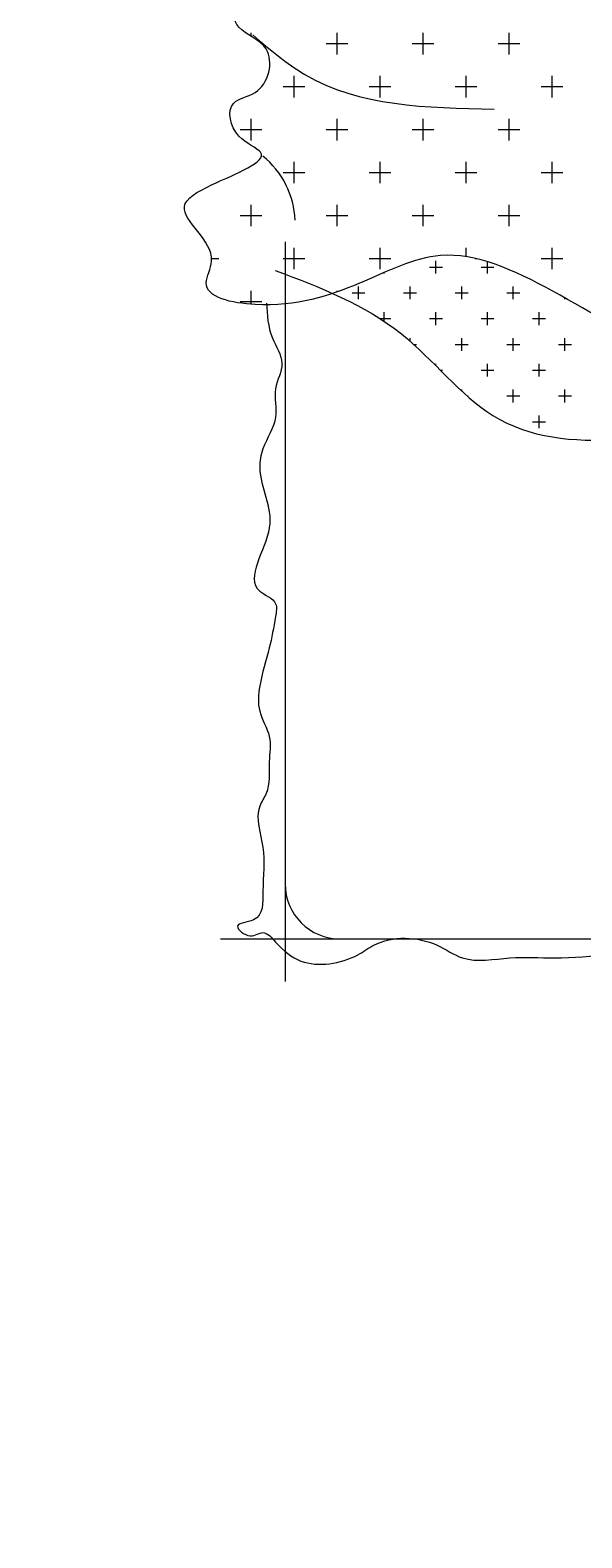
# Model space of a CAD drawing. Units: inches. Extents: x 2330 to 3943, y 1763 to 3461.
# Tile 15 of 40: x 3106 to 3148, y 2547 to 2662. Entities that reach past the tile are written whole.
import ezdxf

# ---------------------------------------------------------------- set-up
doc = ezdxf.new("R2010")
doc.units = ezdxf.units.IN
doc.layers.add('A-ANNO-DIMS', color=2, linetype='Continuous', lineweight=18)
doc.layers.add('A-FURN', color=8, linetype='Continuous', lineweight=13)
doc.styles.get("Standard").update_dxf_attribs({"font": 'arial.ttf'})
doc.dimstyles.get("Standard").update_dxf_attribs({"dimtxt": 0.18, "dimasz": 0.18, "dimexe": 0.18, "dimexo": 0.0625, "dimgap": 0.09, "dimtad": 0, "dimtih": 1, "dimtoh": 1, "dimdec": 4, "dimzin": 0, "dimdsep": 46, "dimtxsty": 'Standard', "dimcen": 0.09, "dimadec": 0, "dimazin": 0, "dimtfac": 1, "dimtdec": 4, "dimtofl": 0, "dimtmove": 0, "dimatfit": 3, "dimfxl": 1, "dimtolj": 1, "dimtzin": 0, "dimarcsym": 0})

# ---------------------------------------------------------------- blocks, each defined once
blk = doc.blocks.new('A$C200C7901')
for p, q in [((0.4504, 1.6834), (0.4504, 1.6883)), ((0.4504, 1.6834), (0.4504, 1.6883)), ((0.4656, 1.6727), (0.466, 1.6727)), ((0.4656, 1.6727), (0.466, 1.6727)), ((0.5597, 1.6727), (0.591, 1.6727)), ((0.5597, 1.6727), (0.591, 1.6727)), ((0.4504, 1.532), (0.4504, 1.5633)), ((0.4347, 1.5477), (0.466, 1.5477)), ((0.6847, 1.5477), (0.716, 1.5477)), ((0.4347, 1.4227), (0.466, 1.4227)), ((0.5, 1.3845), (0.5, 0.3086)), ((0.3931, 1.3602), (0.4035, 1.3602)), ((0.3931, 1.3602), (0.4035, 1.3602)), ((0.4972, 1.3602), (0.5285, 1.3602)), ((0.4972, 1.3602), (0.5285, 1.3602)), ((0.4347, 1.2977), (0.466, 1.2977)), ((0.4347, 1.2977), (0.466, 1.2977)), ((0.4504, 1.2936), (0.4504, 1.3133)), ((0.4504, 1.2936), (0.4504, 1.3133)), ((0.4061, 0.3703), (2.0386, 0.3703))]:
    blk.add_line(p, q)
at = {"linetype": 'ByBlock'}
for p, q in [((0.5754, 1.657), (0.5754, 1.6883)), ((0.5754, 1.657), (0.5754, 1.6883)), ((0.6847, 1.6727), (0.716, 1.6727)), ((0.6847, 1.6727), (0.716, 1.6727)), ((0.7004, 1.657), (0.7004, 1.6883)), ((0.7004, 1.657), (0.7004, 1.6883)), ((0.8097, 1.6727), (0.841, 1.6727)), ((0.8097, 1.6727), (0.841, 1.6727)), ((0.8254, 1.657), (0.8254, 1.6883)), ((0.8254, 1.657), (0.8254, 1.6883)), ((0.5129, 1.5945), (0.5129, 1.6258)), ((0.5129, 1.5945), (0.5129, 1.6258)), ((0.6379, 1.5945), (0.6379, 1.6258)), ((0.6379, 1.5945), (0.6379, 1.6258)), ((0.7629, 1.5945), (0.7629, 1.6258)), ((0.7629, 1.5945), (0.7629, 1.6258)), ((0.8879, 1.5945), (0.8879, 1.6258)), ((0.8879, 1.5945), (0.8879, 1.6258)), ((0.4972, 1.6102), (0.5285, 1.6102)), ((0.4972, 1.6102), (0.5285, 1.6102)), ((0.6222, 1.6102), (0.6535, 1.6102)), ((0.6222, 1.6102), (0.6535, 1.6102)), ((0.7472, 1.6102), (0.7785, 1.6102)), ((0.7472, 1.6102), (0.7785, 1.6102)), ((0.8722, 1.6102), (0.9035, 1.6102)), ((0.8722, 1.6102), (0.9035, 1.6102)), ((0.4504, 1.532), (0.4504, 1.5633)), ((0.5754, 1.532), (0.5754, 1.5633)), ((0.5754, 1.532), (0.5754, 1.5633)), ((0.7004, 1.532), (0.7004, 1.5633)), ((0.7004, 1.532), (0.7004, 1.5633)), ((0.8254, 1.532), (0.8254, 1.5633)), ((0.8254, 1.532), (0.8254, 1.5633)), ((0.4347, 1.5477), (0.466, 1.5477)), ((0.5597, 1.5477), (0.591, 1.5477)), ((0.5597, 1.5477), (0.591, 1.5477)), ((0.6847, 1.5477), (0.716, 1.5477)), ((0.8097, 1.5477), (0.841, 1.5477)), ((0.8097, 1.5477), (0.841, 1.5477)), ((0.5129, 1.4695), (0.5129, 1.5008)), ((0.5129, 1.4695), (0.5129, 1.5008)), ((0.6379, 1.4695), (0.6379, 1.5008)), ((0.6379, 1.4695), (0.6379, 1.5008)), ((0.7629, 1.4695), (0.7629, 1.5008)), ((0.7629, 1.4695), (0.7629, 1.5008)), ((0.8879, 1.4695), (0.8879, 1.5008)), ((0.8879, 1.4695), (0.8879, 1.5008)), ((0.4972, 1.4852), (0.5285, 1.4852)), ((0.4972, 1.4852), (0.5285, 1.4852)), ((0.6222, 1.4852), (0.6535, 1.4852)), ((0.6222, 1.4852), (0.6535, 1.4852)), ((0.7472, 1.4852), (0.7785, 1.4852)), ((0.7472, 1.4852), (0.7785, 1.4852)), ((0.8722, 1.4852), (0.9035, 1.4852)), ((0.8722, 1.4852), (0.9035, 1.4852)), ((0.4504, 1.407), (0.4504, 1.4383)), ((0.4504, 1.407), (0.4504, 1.4383)), ((0.5754, 1.407), (0.5754, 1.4383)), ((0.5754, 1.407), (0.5754, 1.4383)), ((0.7004, 1.407), (0.7004, 1.4383)), ((0.7004, 1.407), (0.7004, 1.4383)), ((0.8254, 1.407), (0.8254, 1.4383)), ((0.8254, 1.407), (0.8254, 1.4383)), ((0.4347, 1.4227), (0.466, 1.4227)), ((0.5597, 1.4227), (0.591, 1.4227)), ((0.5597, 1.4227), (0.591, 1.4227)), ((0.6847, 1.4227), (0.716, 1.4227)), ((0.6847, 1.4227), (0.716, 1.4227)), ((0.8097, 1.4227), (0.841, 1.4227)), ((0.8097, 1.4227), (0.841, 1.4227)), ((0.5129, 1.3445), (0.5129, 1.3758)), ((0.5129, 1.3445), (0.5129, 1.3758)), ((0.6222, 1.3602), (0.6535, 1.3602)), ((0.6222, 1.3602), (0.6535, 1.3602)), ((0.6379, 1.3445), (0.6379, 1.3758)), ((0.6379, 1.3445), (0.6379, 1.3758)), ((0.7629, 1.3627), (0.7629, 1.3758)), ((0.7629, 1.3627), (0.7629, 1.3758)), ((0.7762, 1.3602), (0.7785, 1.3602)), ((0.7762, 1.3602), (0.7785, 1.3602)), ((0.8722, 1.3602), (0.9035, 1.3602)), ((0.8722, 1.3602), (0.9035, 1.3602)), ((0.8879, 1.3445), (0.8879, 1.3758)), ((0.8879, 1.3445), (0.8879, 1.3758)), ((0.6441, 1.3383), (0.6441, 1.3399)), ((0.6441, 1.3383), (0.6441, 1.3399)), ((0.7097, 1.3477), (0.7285, 1.3477)), ((0.7097, 1.3477), (0.7285, 1.3477)), ((0.7191, 1.3383), (0.7191, 1.357)), ((0.7191, 1.3383), (0.7191, 1.357)), ((0.7847, 1.3477), (0.8035, 1.3477)), ((0.7847, 1.3477), (0.8035, 1.3477)), ((0.7941, 1.3383), (0.7941, 1.3554)), ((0.7941, 1.3383), (0.7941, 1.3554)), ((0.6066, 1.3008), (0.6066, 1.3195)), ((0.6066, 1.3008), (0.6066, 1.3195)), ((0.6816, 1.3008), (0.6816, 1.3195)), ((0.6816, 1.3008), (0.6816, 1.3195)), ((0.7566, 1.3008), (0.7566, 1.3195)), ((0.7566, 1.3008), (0.7566, 1.3195)), ((0.8316, 1.3008), (0.8316, 1.3195)), ((0.8316, 1.3008), (0.8316, 1.3195)), ((0.5754, 1.3115), (0.5754, 1.3133)), ((0.5754, 1.3115), (0.5754, 1.3133)), ((0.5972, 1.3102), (0.616, 1.3102)), ((0.5972, 1.3102), (0.616, 1.3102)), ((0.6722, 1.3102), (0.691, 1.3102)), ((0.6722, 1.3102), (0.691, 1.3102)), ((0.7472, 1.3102), (0.766, 1.3102)), ((0.7472, 1.3102), (0.766, 1.3102)), ((0.8222, 1.3102), (0.841, 1.3102)), ((0.8222, 1.3102), (0.841, 1.3102)), ((0.9066, 1.3008), (0.9066, 1.3028)), ((0.9066, 1.3008), (0.9066, 1.3028)), ((0.6379, 1.2727), (0.6535, 1.2727)), ((0.6379, 1.2727), (0.6535, 1.2727)), ((0.6441, 1.2686), (0.6441, 1.282)), ((0.6441, 1.2686), (0.6441, 1.282)), ((0.7097, 1.2727), (0.7285, 1.2727)), ((0.7097, 1.2727), (0.7285, 1.2727)), ((0.7191, 1.2633), (0.7191, 1.282)), ((0.7191, 1.2633), (0.7191, 1.282)), ((0.7847, 1.2727), (0.8035, 1.2727)), ((0.7847, 1.2727), (0.8035, 1.2727)), ((0.7941, 1.2633), (0.7941, 1.282)), ((0.7941, 1.2633), (0.7941, 1.282)), ((0.8597, 1.2727), (0.8785, 1.2727)), ((0.8597, 1.2727), (0.8785, 1.2727)), ((0.8691, 1.2633), (0.8691, 1.282)), ((0.8691, 1.2633), (0.8691, 1.282)), ((0.6816, 1.2398), (0.6816, 1.2445)), ((0.6816, 1.2398), (0.6816, 1.2445)), ((0.6868, 1.2352), (0.691, 1.2352)), ((0.6868, 1.2352), (0.691, 1.2352)), ((0.7472, 1.2352), (0.766, 1.2352)), ((0.7472, 1.2352), (0.766, 1.2352)), ((0.7566, 1.2258), (0.7566, 1.2445)), ((0.7566, 1.2258), (0.7566, 1.2445)), ((0.8222, 1.2352), (0.841, 1.2352)), ((0.8222, 1.2352), (0.841, 1.2352)), ((0.8316, 1.2258), (0.8316, 1.2445)), ((0.8316, 1.2258), (0.8316, 1.2445)), ((0.8972, 1.2352), (0.916, 1.2352)), ((0.8972, 1.2352), (0.916, 1.2352)), ((0.9066, 1.2258), (0.9066, 1.2445)), ((0.9066, 1.2258), (0.9066, 1.2445)), ((0.7191, 1.2041), (0.7191, 1.207)), ((0.7191, 1.2041), (0.7191, 1.207)), ((0.7941, 1.1883), (0.7941, 1.207)), ((0.7941, 1.1883), (0.7941, 1.207)), ((0.8691, 1.1883), (0.8691, 1.207)), ((0.8691, 1.1883), (0.8691, 1.207)), ((0.7255, 1.1977), (0.7285, 1.1977)), ((0.7255, 1.1977), (0.7285, 1.1977)), ((0.7847, 1.1977), (0.8035, 1.1977)), ((0.7847, 1.1977), (0.8035, 1.1977)), ((0.8597, 1.1977), (0.8785, 1.1977)), ((0.8597, 1.1977), (0.8785, 1.1977)), ((0.7566, 1.1674), (0.7566, 1.1695)), ((0.7566, 1.1674), (0.7566, 1.1695)), ((0.8316, 1.1508), (0.8316, 1.1695)), ((0.8316, 1.1508), (0.8316, 1.1695)), ((0.9066, 1.1508), (0.9066, 1.1695)), ((0.9066, 1.1508), (0.9066, 1.1695)), ((0.7646, 1.1602), (0.766, 1.1602)), ((0.7646, 1.1602), (0.766, 1.1602)), ((0.8222, 1.1602), (0.841, 1.1602)), ((0.8222, 1.1602), (0.841, 1.1602)), ((0.8972, 1.1602), (0.916, 1.1602)), ((0.8972, 1.1602), (0.916, 1.1602)), ((0.8597, 1.1227), (0.8785, 1.1227)), ((0.8597, 1.1227), (0.8785, 1.1227)), ((0.8691, 1.1133), (0.8691, 1.132)), ((0.8691, 1.1133), (0.8691, 1.132))]:
    blk.add_line(p, q, dxfattribs=at)
blk.add_arc((0.3888, 1.4113), 0.1256, 1.9962, 51.1646, dxfattribs=at)
for centre, radius, start, end in [((0.3888, 1.4113), 0.1256, 1.9962, 51.1646), ((0.58, 0.4503), 0.08, 180, 270)]:
    blk.add_arc(centre, radius, start, end)
for points, knots in [([(0.4485, 1.7835), (0.4321, 1.7496), (0.4062, 1.6964), (0.49, 1.6713), (0.4719, 1.5969), (0.4123, 1.592), (0.4233, 1.5337), (0.4954, 1.5086), (0.4012, 1.4738), (0.3253, 1.4306), (0.4113, 1.3764), (0.3688, 1.3065), (0.5579, 1.2663), (0.741, 1.4533), (1.1127, 1.1109), (1.4811, 1.2478), (1.7885, 1.3492), (2.0357, 1.1637), (2.0748, 1.2974), (2.0876, 1.349), (2.0192, 1.3805), (2.0564, 1.4298), (2.0588, 1.4846), (1.9759, 1.5349), (2.1004, 1.5845), (2.0397, 1.6519), (1.971, 1.7053), (2.1104, 1.8981), (1.5946, 1.7967), (1.2448, 1.7472), (0.8129, 1.7935), (0.4953, 1.8548), (0.4582, 1.7983), (0.4485, 1.7835)], [0, 0, 0, 0, 88.420092, 139.08588, 204.302936, 239.695496, 287.801042, 327.365471, 412.960499, 463.626286, 552.059846, 584.668336, 662.614915, 940.993281, 1309.926334, 1844.022653, 1996.276242, 2316.43048, 2341.441004, 2404.707416, 2449.463774, 2514.680778, 2538.40571, 2613.031547, 2697.13096, 2760.903931, 2822.692699, 2945.47, 3215.060018, 3725.584917, 4361.974444, 4504.671998, 4555.32777, 4555.32777, 4555.32777, 4555.32777]), ([(0.4856, 1.3429), (0.5504, 1.3182), (0.6715, 1.2721), (0.8374, 1.0498), (1.1164, 1.1183), (1.3878, 1.1816), (1.5888, 1.1102), (1.8403, 1.1127), (1.9415, 1.2178), (2.0032, 1.2819)], [0, 0, 0, 0, 205.411753, 383.654933, 772.067458, 921.644661, 1226.793228, 1388.983508, 1642.292305, 1642.292305, 1642.292305, 1642.292305])]:
    blk.add_open_spline(points, degree=3, knots=knots)
for points, knots in [([(0.4532, 1.6853), (0.4776, 1.6644), (0.574, 1.582), (0.7055, 1.5794), (0.8037, 1.5774)], [0, 0, 0, 0, 94.920667, 374.457292, 374.457292, 374.457292, 374.457292]), ([(0.4532, 1.6853), (0.4776, 1.6644), (0.574, 1.582), (0.7055, 1.5794), (0.8037, 1.5774)], [0, 0, 0, 0, 94.920667, 374.457292, 374.457292, 374.457292, 374.457292]), ([(0.473, 1.2954), (0.4739, 1.2781), (0.4755, 1.2477), (0.5032, 1.2084), (0.4801, 1.1701), (0.4928, 1.1255), (0.4674, 1.0912), (0.4579, 1.0351), (0.501, 0.9724), (0.4311, 0.8832), (0.4902, 0.8637), (0.4843, 0.8288), (0.4774, 0.7906), (0.4625, 0.7457), (0.459, 0.6999), (0.4816, 0.6664), (0.4748, 0.625), (0.4791, 0.5889), (0.4533, 0.5528), (0.4738, 0.5004), (0.4658, 0.4502), (0.4696, 0.3946), (0.4189, 0.3935), (0.4493, 0.3684), (0.4694, 0.3857), (0.4922, 0.3576), (0.5297, 0.3262), (0.5917, 0.3353), (0.6454, 0.3754), (0.7083, 0.3741), (0.7643, 0.3328), (0.826, 0.346), (0.925, 0.3388), (1.0353, 0.3593), (1.1561, 0.3744), (1.2477, 0.3154), (1.3302, 0.3474), (1.4086, 0.3512), (1.5217, 0.3878), (1.6362, 0.3176), (1.7682, 0.3285), (1.8402, 0.3019), (1.9071, 0.3529), (1.9647, 0.3412), (2.0795, 0.2948), (2.0472, 0.3498), (2.0343, 0.3772), (2.0435, 0.43), (2.0109, 0.5782), (2.0746, 0.4643), (2.0805, 0.584), (2.0084, 0.5979), (2.0343, 0.6846), (2.0344, 0.746), (2.0293, 0.8096), (2.0489, 0.8545), (2.0652, 0.9218), (1.9842, 0.9297), (2.0007, 1.0162), (2.0367, 1.0585), (2.0367, 1.1102), (2.0457, 1.1647), (2.0226, 1.2084), (2.0234, 1.2306), (2.0236, 1.2352)], [0, 0, 0, 0, 51.660678, 90.967412, 128.902454, 170.303599, 219.852997, 247.834962, 336.321557, 429.35469, 458.821847, 477.222321, 524.135809, 581.038434, 617.839381, 657.146115, 693.947125, 740.178081, 760.753248, 820.731705, 885.133458, 928.777044, 953.563729, 976.574207, 995.553042, 1018.563482, 1064.584401, 1147.951297, 1174.787598, 1266.851571, 1308.018447, 1377.066427, 1441.511314, 1608.245014, 1714.11869, 1792.771707, 1913.247991, 1954.931389, 2029.864445, 2259.189419, 2305.221512, 2429.507982, 2456.344283, 2543.92595, 2627.925037, 2662.96218, 2687.736879, 2719.937755, 2839.540991, 2875.47895, 2953.681041, 2993.270313, 3066.872333, 3154.395764, 3200.397042, 3248.426375, 3312.828127, 3347.881398, 3444.484026, 3481.577522, 3518.665244, 3592.267265, 3644.719162, 3658.519501, 3658.519501, 3658.519501, 3658.519501])]:
    blk.add_open_spline(points, degree=3, knots=knots, dxfattribs=at)
blk = doc.blocks.new('*D95')
at = {"layer": 'A-ANNO-DIMS', "color": 0, "lineweight": -2, "transparency": 16777216}
for p, q in [((3105.6, 2727.69), (3105.78, 2727.69)), ((3105.69, 2727.6), (3105.69, 2727.78)), ((3606.31, 2659.69), (3418.76, 2685.16))]:
    blk.add_line(p, q, dxfattribs=at)
at = {"layer": 'A-ANNO-DIMS', "color": 0, "transparency": 16777216}
blk.add_solid([(3418.76, 2685.19), (3418.75, 2685.14), (3418.58, 2685.19)], dxfattribs=at)
at = {"layer": 'Defpoints', "color": 0, "transparency": 16777216}
for p in [(3105.69, 2727.69), (3418.58, 2685.19)]:
    blk.add_point(p, dxfattribs=at)
at = {"layer": 'A-ANNO-DIMS', "color": 0, "transparency": 16777216, "insert": (3606.86, 2659.69), "char_height": 0.18, "attachment_point": 5}
blk.add_mtext('\\A1;R315.76', dxfattribs=at)
blk = doc.blocks.new('*D97')
at = {"layer": 'A-ANNO-DIMS', "color": 0, "lineweight": -2, "transparency": 16777216}
for p, q in [((3105.6, 2727.69), (3105.78, 2727.69)), ((3105.69, 2727.6), (3105.69, 2727.78)), ((3589.17, 2615.07), (3408.04, 2657.26))]:
    blk.add_line(p, q, dxfattribs=at)
at = {"layer": 'A-ANNO-DIMS', "color": 0, "transparency": 16777216}
blk.add_solid([(3408.05, 2657.29), (3408.03, 2657.23), (3407.86, 2657.3)], dxfattribs=at)
at = {"layer": 'Defpoints', "color": 0, "transparency": 16777216}
for p in [(3105.69, 2727.69), (3407.86, 2657.3)]:
    blk.add_point(p, dxfattribs=at)
at = {"layer": 'A-ANNO-DIMS', "color": 0, "transparency": 16777216, "insert": (3589.91, 2615.07), "char_height": 0.18, "attachment_point": 5}
blk.add_mtext('\\A1;2X R310.26', dxfattribs=at)
blk = doc.blocks.new('*D98')
at = {"layer": 'A-ANNO-DIMS', "color": 0, "lineweight": -2, "transparency": 16777216}
for p, q in [((3105.6, 2727.69), (3105.78, 2727.69)), ((3105.69, 2727.6), (3105.69, 2727.78)), ((3519.33, 2463.49), (3364.37, 2562.47)), ((3519.51, 2463.49), (3519.33, 2463.49))]:
    blk.add_line(p, q, dxfattribs=at)
at = {"layer": 'A-ANNO-DIMS', "color": 0, "transparency": 16777216}
blk.add_solid([(3364.39, 2562.49), (3364.35, 2562.44), (3364.22, 2562.56)], dxfattribs=at)
at = {"layer": 'Defpoints', "color": 0, "transparency": 16777216}
for p in [(3105.69, 2727.69), (3364.22, 2562.56)]:
    blk.add_point(p, dxfattribs=at)
at = {"layer": 'A-ANNO-DIMS', "color": 0, "transparency": 16777216, "insert": (3520.26, 2463.49), "char_height": 0.18, "attachment_point": 5}
blk.add_mtext('\\A1;3X R306.76', dxfattribs=at)

msp = doc.modelspace()

# ---------------------------------------------------------------- block references
at = {"layer": 'A-FURN', "xscale": 52.5181391560459, "yscale": 52.5181391560459, "zscale": 52.5181391560459}
msp.add_blockref('A$C200C7901', (3098.8053, 2572.8601), dxfattribs=at)

# ---------------------------------------------------------------- dimensions: what is measured, and where the dimension line sits
at = {"layer": 'A-ANNO-DIMS'}
dim = msp.add_radius_dim(center=(3105.6935, 2727.6869), mpoint=(3418.58, 2685.189), dimstyle='Standard', override={"dimdec": 2, "dimlfac": 1, "dimrnd": 0, "dimzin": 0, "dimdsep": 46, "dimlunit": 2}, dxfattribs=at)
dim.commit()
dim.dimension.update_dxf_attribs({"geometry": '*D95', "text_midpoint": (3606.3119, 2659.6902), "dimtype": 164})
for mpoint, text, picture, middle in [((3407.8638, 2657.302), '2X <>', '*D97', (3589.166, 2615.0711)), ((3364.219, 2562.563), '3X <>', '*D98', (3520.2574, 2463.4886))]:
    dim = msp.add_radius_dim(center=(3105.6935, 2727.6869), mpoint=mpoint, text=text, dimstyle='Standard', override={"dimdec": 2, "dimlfac": 1, "dimrnd": 0, "dimzin": 0, "dimdsep": 46, "dimlunit": 2}, dxfattribs=at)
    dim.commit()
    dim.dimension.update_dxf_attribs({"geometry": picture, "text_midpoint": middle, "dimtype": 164})

doc.saveas('drawing.dxf')
